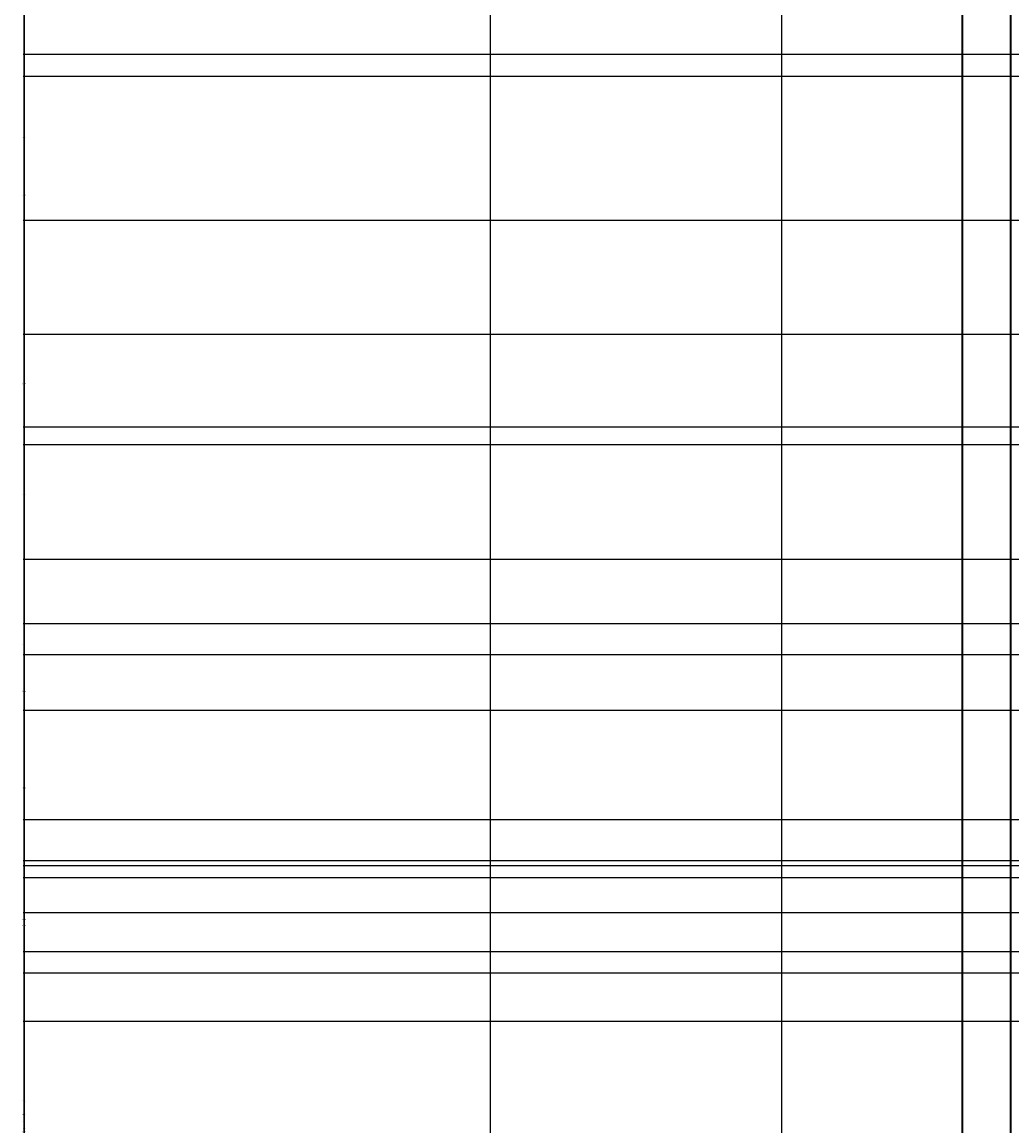
# Model space of a CAD drawing. Units: inches. Extents: x 818 to 1898, y 976 to 2364.
# Tile 9 of 96: x 818 to 1002, y 1668 to 1873. Entities that reach past the tile are written whole.
import ezdxf

# ---------------------------------------------------------------- set-up
doc = ezdxf.new("R2010")
doc.units = ezdxf.units.IN
doc.header["$LTSCALE"] = 5
doc.header["$MEASUREMENT"] = 0
doc.layers.add('A-ANNO-DIMS', color=2, linetype='Continuous', lineweight=18)
doc.layers.add('C-PROP', color=7, linetype='Continuous', lineweight=35)
doc.styles.get("Standard").update_dxf_attribs({"font": 'arial.ttf'})
doc.dimstyles.get("Standard").update_dxf_attribs({"dimtxt": 0.18, "dimasz": 0.18, "dimexe": 0.18, "dimexo": 0.0625, "dimgap": 0.09, "dimtad": 0, "dimtih": 1, "dimtoh": 1, "dimdec": 4, "dimzin": 0, "dimdsep": 46, "dimtxsty": 'Standard', "dimcen": 0.09, "dimadec": 0, "dimazin": 0, "dimtfac": 1, "dimtdec": 4, "dimtofl": 0, "dimtmove": 0, "dimatfit": 3, "dimfxl": 1, "dimtolj": 1, "dimtzin": 0, "dimarcsym": 0})

# ---------------------------------------------------------------- blocks, each defined once
blk = doc.blocks.new('*D59')
at = {"layer": 'A-ANNO-DIMS', "color": 0, "lineweight": -2, "ltscale": 5, "transparency": 16777216}
for p, q in [((1251.64, 2300.39), (818.03, 2300.39)), ((818.21, 2300.21), (818.21, 1669.95)), ((818.21, 1039.32), (818.21, 1669.59)), ((896.05, 1039.14), (818.03, 1039.14))]:
    blk.add_line(p, q, dxfattribs=at)
at = {"layer": 'A-ANNO-DIMS', "color": 0, "ltscale": 5, "transparency": 16777216}
for points in [[(818.18, 2300.21), (818.24, 2300.21), (818.21, 2300.39)], [(818.18, 1039.32), (818.24, 1039.32), (818.21, 1039.14)]]:
    blk.add_solid(points, dxfattribs=at)
at = {"layer": 'Defpoints', "color": 0, "ltscale": 5, "transparency": 16777216}
for p in [(818.21, 2300.39), (1251.71, 2300.39), (896.11, 1039.14)]:
    blk.add_point(p, dxfattribs=at)
at = {"layer": 'A-ANNO-DIMS', "color": 0, "ltscale": 5, "transparency": 16777216, "insert": (818.21, 1669.77), "char_height": 0.18, "attachment_point": 5}
blk.add_mtext('\\A1;1261.2', dxfattribs=at)
blk = doc.blocks.new('*D60')
at = {"layer": 'A-ANNO-DIMS', "color": 0, "lineweight": -2, "ltscale": 5, "transparency": 16777216}
for p, q in [((992.66, 2294.22), (818.03, 2294.22)), ((818.21, 2294.04), (818.21, 1748.77)), ((818.21, 1203.14), (818.21, 1748.41)), ((992.66, 1202.96), (818.03, 1202.96))]:
    blk.add_line(p, q, dxfattribs=at)
at = {"layer": 'A-ANNO-DIMS', "color": 0, "ltscale": 5, "transparency": 16777216}
for points in [[(818.18, 2294.04), (818.24, 2294.04), (818.21, 2294.22)], [(818.18, 1203.14), (818.24, 1203.14), (818.21, 1202.96)]]:
    blk.add_solid(points, dxfattribs=at)
at = {"layer": 'Defpoints', "color": 0, "ltscale": 5, "transparency": 16777216}
for p in [(818.21, 2294.22), (992.73, 2294.22), (992.73, 1202.96)]:
    blk.add_point(p, dxfattribs=at)
at = {"layer": 'A-ANNO-DIMS', "color": 0, "ltscale": 5, "transparency": 16777216, "insert": (818.21, 1748.59), "char_height": 0.18, "attachment_point": 5}
blk.add_mtext('\\A1;1091.3', dxfattribs=at)
blk = doc.blocks.new('*D79')
at = {"layer": 'A-ANNO-DIMS', "color": 0, "lineweight": -2, "ltscale": 5, "transparency": 16777216}
for p, q in [((992.73, 1203.03), (992.73, 2363.87)), ((992.91, 2363.69), (1032.01, 2363.69)), ((1071.55, 2363.69), (1032.44, 2363.69)), ((1071.73, 1203.03), (1071.73, 2363.87))]:
    blk.add_line(p, q, dxfattribs=at)
at = {"layer": 'A-ANNO-DIMS', "color": 0, "ltscale": 5, "transparency": 16777216}
for points in [[(992.91, 2363.72), (992.91, 2363.66), (992.73, 2363.69)], [(1071.55, 2363.72), (1071.55, 2363.66), (1071.73, 2363.69)]]:
    blk.add_solid(points, dxfattribs=at)
at = {"layer": 'Defpoints', "color": 0, "ltscale": 5, "transparency": 16777216}
for p in [(1071.73, 2363.69), (992.73, 1202.96), (1071.73, 1202.96)]:
    blk.add_point(p, dxfattribs=at)
at = {"layer": 'A-ANNO-DIMS', "color": 0, "ltscale": 5, "transparency": 16777216, "insert": (1032.23, 2363.69), "char_height": 0.18, "attachment_point": 5}
blk.add_mtext('\\A1;79', dxfattribs=at)
blk = doc.blocks.new('*D84')
at = {"layer": 'A-ANNO-DIMS', "color": 0, "lineweight": -2, "ltscale": 5, "transparency": 16777216}
for p, q in [((1197.66, 1700.08), (818.03, 1700.08)), ((818.21, 1699.9), (818.21, 1600.76)), ((818.21, 1501.26), (818.21, 1600.4)), ((1197.66, 1501.08), (818.03, 1501.08))]:
    blk.add_line(p, q, dxfattribs=at)
at = {"layer": 'A-ANNO-DIMS', "color": 0, "ltscale": 5, "transparency": 16777216}
for points in [[(818.18, 1699.9), (818.24, 1699.9), (818.21, 1700.08)], [(818.18, 1501.26), (818.24, 1501.26), (818.21, 1501.08)]]:
    blk.add_solid(points, dxfattribs=at)
at = {"layer": 'Defpoints', "color": 0, "ltscale": 5, "transparency": 16777216}
for p in [(818.21, 1700.08), (1197.73, 1700.08), (1197.73, 1501.08)]:
    blk.add_point(p, dxfattribs=at)
at = {"layer": 'A-ANNO-DIMS', "color": 0, "ltscale": 5, "transparency": 16777216, "insert": (818.21, 1600.58), "char_height": 0.18, "attachment_point": 5}
blk.add_mtext('\\A1;199', dxfattribs=at)
blk = doc.blocks.new('*D90')
at = {"layer": 'A-ANNO-DIMS', "color": 0, "lineweight": -2, "ltscale": 5, "transparency": 16777216}
for p, q in [((904.95, 1071.12), (904.95, 2363.87)), ((905.13, 2363.69), (931.67, 2363.69)), ((958.99, 2363.69), (932.45, 2363.69)), ((959.17, 1071.12), (959.17, 2363.87))]:
    blk.add_line(p, q, dxfattribs=at)
at = {"layer": 'A-ANNO-DIMS', "color": 0, "ltscale": 5, "transparency": 16777216}
for points in [[(905.13, 2363.72), (905.13, 2363.66), (904.95, 2363.69)], [(958.99, 2363.72), (958.99, 2363.66), (959.17, 2363.69)]]:
    blk.add_solid(points, dxfattribs=at)
at = {"layer": 'Defpoints', "color": 0, "ltscale": 5, "transparency": 16777216}
for p in [(959.17, 2363.69), (904.95, 1071.06), (959.17, 1071.06)]:
    blk.add_point(p, dxfattribs=at)
at = {"layer": 'A-ANNO-DIMS', "color": 0, "ltscale": 5, "transparency": 16777216, "insert": (932.06, 2363.69), "char_height": 0.18, "attachment_point": 5}
blk.add_mtext('\\A1;54.22', dxfattribs=at)
blk = doc.blocks.new('*D91')
at = {"layer": 'A-ANNO-DIMS', "color": 0, "lineweight": -2, "ltscale": 5, "transparency": 16777216}
for p, q in [((959.17, 1071.12), (959.17, 2363.87)), ((959.35, 2363.69), (985.8, 2363.69)), ((1013.04, 2363.69), (986.59, 2363.69)), ((1013.22, 1071.12), (1013.22, 2363.87))]:
    blk.add_line(p, q, dxfattribs=at)
at = {"layer": 'A-ANNO-DIMS', "color": 0, "ltscale": 5, "transparency": 16777216}
for points in [[(959.35, 2363.72), (959.35, 2363.66), (959.17, 2363.69)], [(1013.04, 2363.72), (1013.04, 2363.66), (1013.22, 2363.69)]]:
    blk.add_solid(points, dxfattribs=at)
at = {"layer": 'Defpoints', "color": 0, "ltscale": 5, "transparency": 16777216}
for p in [(1013.22, 2363.69), (959.17, 1071.06), (1013.22, 1071.06)]:
    blk.add_point(p, dxfattribs=at)
at = {"layer": 'A-ANNO-DIMS', "color": 0, "ltscale": 5, "transparency": 16777216, "insert": (986.2, 2363.69), "char_height": 0.18, "attachment_point": 5}
blk.add_mtext('\\A1;54.04', dxfattribs=at)
blk = doc.blocks.new('*D119')
at = {"layer": 'A-ANNO-DIMS', "color": 0, "lineweight": -2, "ltscale": 5, "transparency": 16777216}
for p, q in [((1766.29, 1716.99), (818.03, 1716.99)), ((818.21, 1716.81), (818.21, 1672.43)), ((818.21, 1627.69), (818.21, 1672.06)), ((1766.29, 1627.51), (818.03, 1627.51))]:
    blk.add_line(p, q, dxfattribs=at)
at = {"layer": 'A-ANNO-DIMS', "color": 0, "ltscale": 5, "transparency": 16777216}
for points in [[(818.18, 1716.81), (818.24, 1716.81), (818.21, 1716.99)], [(818.18, 1627.69), (818.24, 1627.69), (818.21, 1627.51)]]:
    blk.add_solid(points, dxfattribs=at)
at = {"layer": 'Defpoints', "color": 0, "ltscale": 5, "transparency": 16777216}
for p in [(818.21, 1716.99), (1766.35, 1716.99), (1766.35, 1627.51)]:
    blk.add_point(p, dxfattribs=at)
at = {"layer": 'A-ANNO-DIMS', "color": 0, "ltscale": 5, "transparency": 16777216, "insert": (818.21, 1672.25), "char_height": 0.18, "attachment_point": 5}
blk.add_mtext('\\A1;89.48', dxfattribs=at)
blk = doc.blocks.new('*D120')
at = {"layer": 'A-ANNO-DIMS', "color": 0, "lineweight": -2, "ltscale": 5, "transparency": 16777216}
for p, q in [((1766.29, 1797.72), (818.03, 1797.72)), ((818.21, 1797.54), (818.21, 1757.53)), ((818.21, 1717.17), (818.21, 1757.17)), ((1766.29, 1716.99), (818.03, 1716.99))]:
    blk.add_line(p, q, dxfattribs=at)
at = {"layer": 'A-ANNO-DIMS', "color": 0, "ltscale": 5, "transparency": 16777216}
for points in [[(818.18, 1797.54), (818.24, 1797.54), (818.21, 1797.72)], [(818.18, 1717.17), (818.24, 1717.17), (818.21, 1716.99)]]:
    blk.add_solid(points, dxfattribs=at)
at = {"layer": 'Defpoints', "color": 0, "ltscale": 5, "transparency": 16777216}
for p in [(818.21, 1797.72), (1766.35, 1797.72), (1766.35, 1716.99)]:
    blk.add_point(p, dxfattribs=at)
at = {"layer": 'A-ANNO-DIMS', "color": 0, "ltscale": 5, "transparency": 16777216, "insert": (818.21, 1757.35), "char_height": 0.18, "attachment_point": 5}
blk.add_mtext('\\A1;80.73', dxfattribs=at)
blk = doc.blocks.new('*D121')
at = {"layer": 'A-ANNO-DIMS', "color": 0, "lineweight": -2, "ltscale": 5, "transparency": 16777216}
for p, q in [((1766.29, 1884.2), (818.03, 1884.2)), ((818.21, 1884.02), (818.21, 1841.14)), ((818.21, 1797.9), (818.21, 1840.78)), ((1766.29, 1797.72), (818.03, 1797.72))]:
    blk.add_line(p, q, dxfattribs=at)
at = {"layer": 'A-ANNO-DIMS', "color": 0, "ltscale": 5, "transparency": 16777216}
for points in [[(818.18, 1884.02), (818.24, 1884.02), (818.21, 1884.2)], [(818.18, 1797.9), (818.24, 1797.9), (818.21, 1797.72)]]:
    blk.add_solid(points, dxfattribs=at)
at = {"layer": 'Defpoints', "color": 0, "ltscale": 5, "transparency": 16777216}
for p in [(818.21, 1884.2), (1766.35, 1884.2), (1766.35, 1797.72)]:
    blk.add_point(p, dxfattribs=at)
at = {"layer": 'A-ANNO-DIMS', "color": 0, "ltscale": 5, "transparency": 16777216, "insert": (818.21, 1840.96), "char_height": 0.18, "attachment_point": 5}
blk.add_mtext('\\A1;86.49', dxfattribs=at)
blk = doc.blocks.new('*D124')
at = {"layer": 'A-ANNO-DIMS', "color": 0, "lineweight": -2, "ltscale": 5, "transparency": 16777216}
for p, q in [((1131.7, 1974.57), (818.03, 1974.57)), ((818.21, 1974.39), (818.21, 1884.68)), ((818.21, 1794.61), (818.21, 1884.32)), ((1138.44, 1794.43), (818.03, 1794.43))]:
    blk.add_line(p, q, dxfattribs=at)
at = {"layer": 'A-ANNO-DIMS', "color": 0, "ltscale": 5, "transparency": 16777216}
for points in [[(818.18, 1974.39), (818.24, 1974.39), (818.21, 1974.57)], [(818.18, 1794.61), (818.24, 1794.61), (818.21, 1794.43)]]:
    blk.add_solid(points, dxfattribs=at)
at = {"layer": 'Defpoints', "color": 0, "ltscale": 5, "transparency": 16777216}
for p in [(818.21, 1974.57), (1131.77, 1974.57), (1138.5, 1794.43)]:
    blk.add_point(p, dxfattribs=at)
at = {"layer": 'A-ANNO-DIMS', "color": 0, "ltscale": 5, "transparency": 16777216, "insert": (818.21, 1884.5), "char_height": 0.18, "attachment_point": 5}
blk.add_mtext('\\A1;180.14', dxfattribs=at)
blk = doc.blocks.new('*D130')
at = {"layer": 'A-ANNO-DIMS', "color": 0, "lineweight": -2, "ltscale": 5, "transparency": 16777216}
for p, q in [((1044.78, 1724.63), (818.03, 1724.63)), ((818.21, 1724.45), (818.21, 1666.75)), ((818.21, 1608.69), (818.21, 1666.39)), ((1044.78, 1608.51), (818.03, 1608.51))]:
    blk.add_line(p, q, dxfattribs=at)
at = {"layer": 'A-ANNO-DIMS', "color": 0, "ltscale": 5, "transparency": 16777216}
for points in [[(818.18, 1724.45), (818.24, 1724.45), (818.21, 1724.63)], [(818.18, 1608.69), (818.24, 1608.69), (818.21, 1608.51)]]:
    blk.add_solid(points, dxfattribs=at)
at = {"layer": 'Defpoints', "color": 0, "ltscale": 5, "transparency": 16777216}
for p in [(818.21, 1724.63), (1044.85, 1724.63), (1044.85, 1608.51)]:
    blk.add_point(p, dxfattribs=at)
at = {"layer": 'A-ANNO-DIMS', "color": 0, "ltscale": 5, "transparency": 16777216, "insert": (818.21, 1666.57), "char_height": 0.18, "attachment_point": 5}
blk.add_mtext('\\A1;116.12', dxfattribs=at)
blk = doc.blocks.new('*D131')
at = {"layer": 'A-ANNO-DIMS', "color": 0, "lineweight": -2, "ltscale": 5, "transparency": 16777216}
for p, q in [((1043.71, 1886.9), (818.03, 1886.9)), ((818.21, 1886.72), (818.21, 1805.95)), ((818.21, 1724.81), (818.21, 1805.58)), ((1044.78, 1724.63), (818.03, 1724.63))]:
    blk.add_line(p, q, dxfattribs=at)
at = {"layer": 'A-ANNO-DIMS', "color": 0, "ltscale": 5, "transparency": 16777216}
for points in [[(818.18, 1886.72), (818.24, 1886.72), (818.21, 1886.9)], [(818.18, 1724.81), (818.24, 1724.81), (818.21, 1724.63)]]:
    blk.add_solid(points, dxfattribs=at)
at = {"layer": 'Defpoints', "color": 0, "ltscale": 5, "transparency": 16777216}
for p in [(818.21, 1886.9), (1043.77, 1886.9), (1044.85, 1724.63)]:
    blk.add_point(p, dxfattribs=at)
at = {"layer": 'A-ANNO-DIMS', "color": 0, "ltscale": 5, "transparency": 16777216, "insert": (818.21, 1805.77), "char_height": 0.18, "attachment_point": 5}
blk.add_mtext('\\A1;162.27', dxfattribs=at)
blk = doc.blocks.new('*D162')
at = {"layer": 'A-ANNO-DIMS', "color": 0, "lineweight": -2, "ltscale": 5, "transparency": 16777216}
for p, q in [((1429.16, 1876.08), (818.03, 1876.08)), ((818.21, 1875.9), (818.21, 1871.76)), ((818.21, 1867.26), (818.21, 1871.4)), ((1429.16, 1867.08), (818.03, 1867.08))]:
    blk.add_line(p, q, dxfattribs=at)
at = {"layer": 'A-ANNO-DIMS', "color": 0, "ltscale": 5, "transparency": 16777216}
for points in [[(818.18, 1875.9), (818.24, 1875.9), (818.21, 1876.08)], [(818.18, 1867.26), (818.24, 1867.26), (818.21, 1867.08)]]:
    blk.add_solid(points, dxfattribs=at)
at = {"layer": 'Defpoints', "color": 0, "ltscale": 5, "transparency": 16777216}
for p in [(1429.23, 1876.08), (818.21, 1867.08), (1429.23, 1867.08)]:
    blk.add_point(p, dxfattribs=at)
at = {"layer": 'A-ANNO-DIMS', "color": 0, "ltscale": 5, "transparency": 16777216, "insert": (818.21, 1871.58), "char_height": 0.18, "attachment_point": 5}
blk.add_mtext('\\A1;9', dxfattribs=at)
blk = doc.blocks.new('*D176')
at = {"layer": 'A-ANNO-DIMS', "color": 0, "lineweight": -2, "ltscale": 5, "transparency": 16777216}
for p, q in [((1559.66, 1687.08), (818.03, 1687.08)), ((818.21, 1686.9), (818.21, 1667.51)), ((818.21, 1647.76), (818.21, 1667.15)), ((1559.66, 1647.58), (818.03, 1647.58))]:
    blk.add_line(p, q, dxfattribs=at)
at = {"layer": 'A-ANNO-DIMS', "color": 0, "ltscale": 5, "transparency": 16777216}
for points in [[(818.18, 1686.9), (818.24, 1686.9), (818.21, 1687.08)], [(818.18, 1647.76), (818.24, 1647.76), (818.21, 1647.58)]]:
    blk.add_solid(points, dxfattribs=at)
at = {"layer": 'Defpoints', "color": 0, "ltscale": 5, "transparency": 16777216}
for p in [(1559.73, 1687.08), (818.21, 1647.58), (1559.73, 1647.58)]:
    blk.add_point(p, dxfattribs=at)
at = {"layer": 'A-ANNO-DIMS', "color": 0, "ltscale": 5, "transparency": 16777216, "insert": (818.21, 1667.33), "char_height": 0.18, "attachment_point": 5}
blk.add_mtext('\\A1;39.5', dxfattribs=at)
blk = doc.blocks.new('*D215')
at = {"layer": 'A-ANNO-DIMS', "color": 0, "lineweight": -2, "ltscale": 5, "transparency": 16777216}
for p, q in [((1590.66, 1876.08), (818.03, 1876.08)), ((818.21, 1875.9), (818.21, 1781.76)), ((818.21, 1687.26), (818.21, 1781.4)), ((1511.66, 1687.08), (818.03, 1687.08))]:
    blk.add_line(p, q, dxfattribs=at)
at = {"layer": 'A-ANNO-DIMS', "color": 0, "ltscale": 5, "transparency": 16777216}
for points in [[(818.18, 1875.9), (818.24, 1875.9), (818.21, 1876.08)], [(818.18, 1687.26), (818.24, 1687.26), (818.21, 1687.08)]]:
    blk.add_solid(points, dxfattribs=at)
at = {"layer": 'Defpoints', "color": 0, "ltscale": 5, "transparency": 16777216}
for p in [(818.21, 1876.08), (1590.73, 1876.08), (1511.73, 1687.08)]:
    blk.add_point(p, dxfattribs=at)
at = {"layer": 'A-ANNO-DIMS', "color": 0, "ltscale": 5, "transparency": 16777216, "insert": (818.21, 1781.58), "char_height": 0.18, "attachment_point": 5}
blk.add_mtext('\\A1;189', dxfattribs=at)
blk = doc.blocks.new('*D220')
at = {"layer": 'A-ANNO-DIMS', "color": 0, "lineweight": -2, "ltscale": 5, "transparency": 16777216}
for p, q in [((1520.66, 1773.08), (818.03, 1773.08)), ((818.21, 1772.9), (818.21, 1767.26)), ((818.21, 1761.26), (818.21, 1766.9)), ((1520.66, 1761.08), (818.03, 1761.08))]:
    blk.add_line(p, q, dxfattribs=at)
at = {"layer": 'A-ANNO-DIMS', "color": 0, "ltscale": 5, "transparency": 16777216}
for points in [[(818.18, 1772.9), (818.24, 1772.9), (818.21, 1773.08)], [(818.18, 1761.26), (818.24, 1761.26), (818.21, 1761.08)]]:
    blk.add_solid(points, dxfattribs=at)
at = {"layer": 'Defpoints', "color": 0, "ltscale": 5, "transparency": 16777216}
for p in [(818.21, 1773.08), (1520.73, 1773.08), (1520.73, 1761.08)]:
    blk.add_point(p, dxfattribs=at)
at = {"layer": 'A-ANNO-DIMS', "color": 0, "ltscale": 5, "transparency": 16777216, "insert": (818.21, 1767.08), "char_height": 0.18, "attachment_point": 5}
blk.add_mtext('\\A1;12', dxfattribs=at)
blk = doc.blocks.new('*D222')
at = {"layer": 'A-ANNO-DIMS', "color": 0, "lineweight": -2, "ltscale": 5, "transparency": 16777216}
for p, q in [((1511.66, 1744.97), (818.03, 1744.97)), ((818.21, 1744.79), (818.21, 1730.69)), ((818.21, 1716.23), (818.21, 1730.33)), ((1511.66, 1716.05), (818.03, 1716.05))]:
    blk.add_line(p, q, dxfattribs=at)
at = {"layer": 'A-ANNO-DIMS', "color": 0, "ltscale": 5, "transparency": 16777216}
for points in [[(818.18, 1744.79), (818.24, 1744.79), (818.21, 1744.97)], [(818.18, 1716.23), (818.24, 1716.23), (818.21, 1716.05)]]:
    blk.add_solid(points, dxfattribs=at)
at = {"layer": 'Defpoints', "color": 0, "ltscale": 5, "transparency": 16777216}
for p in [(818.21, 1744.97), (1511.73, 1744.97), (1511.73, 1716.05)]:
    blk.add_point(p, dxfattribs=at)
at = {"layer": 'A-ANNO-DIMS', "color": 0, "ltscale": 5, "transparency": 16777216, "insert": (818.21, 1730.51), "char_height": 0.18, "attachment_point": 5}
blk.add_mtext('\\A1;28.926', dxfattribs=at)
blk = doc.blocks.new('*D223')
at = {"layer": 'A-ANNO-DIMS', "color": 0, "lineweight": -2, "ltscale": 5, "transparency": 16777216}
for p, q in [((1511.66, 1716.05), (818.03, 1716.05)), ((818.21, 1715.87), (818.21, 1706.24)), ((818.21, 1696.26), (818.21, 1705.88)), ((1511.66, 1696.08), (818.03, 1696.08))]:
    blk.add_line(p, q, dxfattribs=at)
at = {"layer": 'A-ANNO-DIMS', "color": 0, "ltscale": 5, "transparency": 16777216}
for points in [[(818.18, 1715.87), (818.24, 1715.87), (818.21, 1716.05)], [(818.18, 1696.26), (818.24, 1696.26), (818.21, 1696.08)]]:
    blk.add_solid(points, dxfattribs=at)
at = {"layer": 'Defpoints', "color": 0, "ltscale": 5, "transparency": 16777216}
for p in [(818.21, 1716.05), (1511.73, 1716.05), (1511.73, 1696.08)]:
    blk.add_point(p, dxfattribs=at)
at = {"layer": 'A-ANNO-DIMS', "color": 0, "ltscale": 5, "transparency": 16777216, "insert": (818.21, 1706.06), "char_height": 0.18, "attachment_point": 5}
blk.add_mtext('\\A1;19.967', dxfattribs=at)
blk = doc.blocks.new('*D227')
at = {"layer": 'A-ANNO-DIMS', "color": 0, "lineweight": -2, "ltscale": 5, "transparency": 16777216}
for p, q in [((1595.66, 1867.08), (818.03, 1867.08)), ((818.21, 1866.9), (818.21, 1851.81)), ((818.21, 1836.36), (818.21, 1851.45)), ((1594.66, 1836.18), (818.03, 1836.18))]:
    blk.add_line(p, q, dxfattribs=at)
at = {"layer": 'A-ANNO-DIMS', "color": 0, "ltscale": 5, "transparency": 16777216}
for points in [[(818.18, 1866.9), (818.24, 1866.9), (818.21, 1867.08)], [(818.18, 1836.36), (818.24, 1836.36), (818.21, 1836.18)]]:
    blk.add_solid(points, dxfattribs=at)
at = {"layer": 'Defpoints', "color": 0, "ltscale": 5, "transparency": 16777216}
for p in [(818.21, 1867.08), (1595.73, 1867.08), (1594.73, 1836.18)]:
    blk.add_point(p, dxfattribs=at)
at = {"layer": 'A-ANNO-DIMS', "color": 0, "ltscale": 5, "transparency": 16777216, "insert": (818.21, 1851.63), "char_height": 0.18, "attachment_point": 5}
blk.add_mtext('\\A1;30.894', dxfattribs=at)
blk = doc.blocks.new('*D246')
at = {"layer": 'A-ANNO-DIMS', "color": 0, "lineweight": -2, "ltscale": 5, "transparency": 16777216}
for p, q in [((1258.66, 1755.33), (818.03, 1755.33)), ((818.21, 1755.15), (818.21, 1731.51)), ((818.21, 1707.51), (818.21, 1731.15)), ((1258.66, 1707.33), (818.03, 1707.33))]:
    blk.add_line(p, q, dxfattribs=at)
at = {"layer": 'A-ANNO-DIMS', "color": 0, "ltscale": 5, "transparency": 16777216}
for points in [[(818.18, 1755.15), (818.24, 1755.15), (818.21, 1755.33)], [(818.18, 1707.51), (818.24, 1707.51), (818.21, 1707.33)]]:
    blk.add_solid(points, dxfattribs=at)
at = {"layer": 'Defpoints', "color": 0, "ltscale": 5, "transparency": 16777216}
for p in [(818.21, 1755.33), (1258.73, 1755.33), (1258.73, 1707.33)]:
    blk.add_point(p, dxfattribs=at)
at = {"layer": 'A-ANNO-DIMS', "color": 0, "ltscale": 5, "transparency": 16777216, "insert": (818.21, 1731.33), "char_height": 0.18, "attachment_point": 5}
blk.add_mtext('\\A1;48', dxfattribs=at)
blk = doc.blocks.new('*D247')
at = {"layer": 'A-ANNO-DIMS', "color": 0, "lineweight": -2, "ltscale": 5, "transparency": 16777216}
for p, q in [((1258.66, 1862.97), (818.03, 1862.97)), ((818.21, 1862.79), (818.21, 1839.15)), ((818.21, 1815.15), (818.21, 1838.78)), ((1258.66, 1814.97), (818.03, 1814.97))]:
    blk.add_line(p, q, dxfattribs=at)
at = {"layer": 'A-ANNO-DIMS', "color": 0, "ltscale": 5, "transparency": 16777216}
for points in [[(818.18, 1862.79), (818.24, 1862.79), (818.21, 1862.97)], [(818.18, 1815.15), (818.24, 1815.15), (818.21, 1814.97)]]:
    blk.add_solid(points, dxfattribs=at)
at = {"layer": 'Defpoints', "color": 0, "ltscale": 5, "transparency": 16777216}
for p in [(818.21, 1862.97), (1258.73, 1862.97), (1258.73, 1814.97)]:
    blk.add_point(p, dxfattribs=at)
at = {"layer": 'A-ANNO-DIMS', "color": 0, "ltscale": 5, "transparency": 16777216, "insert": (818.21, 1838.97), "char_height": 0.18, "attachment_point": 5}
blk.add_mtext('\\A1;48', dxfattribs=at)
blk = doc.blocks.new('*D249')
at = {"layer": 'A-ANNO-DIMS', "color": 0, "lineweight": -2, "ltscale": 5, "transparency": 16777216}
for p, q in [((1258.66, 1814.97), (818.03, 1814.97)), ((818.21, 1814.79), (818.21, 1785.33)), ((818.21, 1755.51), (818.21, 1784.97)), ((1258.66, 1755.33), (818.03, 1755.33))]:
    blk.add_line(p, q, dxfattribs=at)
at = {"layer": 'A-ANNO-DIMS', "color": 0, "ltscale": 5, "transparency": 16777216}
for points in [[(818.18, 1814.79), (818.24, 1814.79), (818.21, 1814.97)], [(818.18, 1755.51), (818.24, 1755.51), (818.21, 1755.33)]]:
    blk.add_solid(points, dxfattribs=at)
at = {"layer": 'Defpoints', "color": 0, "ltscale": 5, "transparency": 16777216}
for p in [(818.21, 1814.97), (1258.73, 1814.97), (1258.73, 1755.33)]:
    blk.add_point(p, dxfattribs=at)
at = {"layer": 'A-ANNO-DIMS', "color": 0, "ltscale": 5, "transparency": 16777216, "insert": (818.21, 1785.15), "char_height": 0.18, "attachment_point": 5}
blk.add_mtext('\\A1;59.63', dxfattribs=at)
blk = doc.blocks.new('*D277')
at = {"layer": 'A-ANNO-DIMS', "color": 0, "lineweight": -2, "ltscale": 5, "transparency": 16777216}
for p, q in [((1251.87, 1687.08), (818.03, 1687.08)), ((818.21, 1686.9), (818.21, 1668.7)), ((818.21, 1650.13), (818.21, 1668.33)), ((1256.59, 1649.95), (818.03, 1649.95))]:
    blk.add_line(p, q, dxfattribs=at)
at = {"layer": 'A-ANNO-DIMS', "color": 0, "ltscale": 5, "transparency": 16777216}
for points in [[(818.18, 1686.9), (818.24, 1686.9), (818.21, 1687.08)], [(818.18, 1650.13), (818.24, 1650.13), (818.21, 1649.95)]]:
    blk.add_solid(points, dxfattribs=at)
at = {"layer": 'Defpoints', "color": 0, "ltscale": 5, "transparency": 16777216}
for p in [(818.21, 1687.08), (1251.93, 1687.08), (1256.65, 1649.95)]:
    blk.add_point(p, dxfattribs=at)
at = {"layer": 'A-ANNO-DIMS', "color": 0, "ltscale": 5, "transparency": 16777216, "insert": (818.21, 1668.52), "char_height": 0.18, "attachment_point": 5}
blk.add_mtext('\\A1;37.13', dxfattribs=at)
blk = doc.blocks.new('*D289')
at = {"layer": 'A-ANNO-DIMS', "color": 0, "lineweight": -2, "ltscale": 5, "transparency": 16777216}
for p, q in [((1279.06, 1713.82), (818.03, 1713.82)), ((818.21, 1713.64), (818.21, 1705.13)), ((818.21, 1696.26), (818.21, 1704.77)), ((1267.66, 1696.08), (818.03, 1696.08))]:
    blk.add_line(p, q, dxfattribs=at)
at = {"layer": 'A-ANNO-DIMS', "color": 0, "ltscale": 5, "transparency": 16777216}
for points in [[(818.18, 1713.64), (818.24, 1713.64), (818.21, 1713.82)], [(818.18, 1696.26), (818.24, 1696.26), (818.21, 1696.08)]]:
    blk.add_solid(points, dxfattribs=at)
at = {"layer": 'Defpoints', "color": 0, "ltscale": 5, "transparency": 16777216}
for p in [(1279.13, 1713.82), (818.21, 1696.08), (1267.73, 1696.08)]:
    blk.add_point(p, dxfattribs=at)
at = {"layer": 'A-ANNO-DIMS', "color": 0, "ltscale": 5, "transparency": 16777216, "insert": (818.21, 1704.95), "char_height": 0.18, "attachment_point": 5}
blk.add_mtext('\\A1;17.74', dxfattribs=at)

msp = doc.modelspace()

# ---------------------------------------------------------------- linework, layer by layer
at = {"layer": 'C-PROP'}
for p, q in [((992.7251, 2294.2171), (992.7251, 1202.9642)), ((1001.7252, 2285.2171), (1001.7252, 1211.9642))]:
    msp.add_line(p, q, dxfattribs=at)

# ---------------------------------------------------------------- dimensions: what is measured, and where the dimension line sits
at = {"layer": 'A-ANNO-DIMS', "ltscale": 5}
for base, p1, p2, override, picture, middle in [((959.1737, 2363.6929), (904.9504, 1071.0552), (959.1737, 1071.0552), {"dimdec": 2, "dimlfac": 1, "dimrnd": 0, "dimzin": 0, "dimdsep": 46, "dimlunit": 2}, '*D90', (932.062, 2363.6929)), ((1013.2176, 2363.6929), (959.1737, 1071.0552), (1013.2176, 1071.0552), {"dimdec": 2, "dimlfac": 1, "dimrnd": 0, "dimzin": 0, "dimdsep": 46, "dimlunit": 2}, '*D91', (986.1956, 2363.6929)), ((1071.7251, 2363.6929), (992.7251, 1202.9642), (1071.7251, 1202.9642), {"dimdec": 0, "dimlfac": 1, "dimrnd": 0, "dimzin": 0, "dimdsep": 46, "dimlunit": 2}, '*D79', (1032.2251, 2363.6929))]:
    dim = msp.add_linear_dim(base=base, p1=p1, p2=p2, dimstyle='Standard', override=override, dxfattribs=at)
    dim.commit()
    dim.dimension.update_dxf_attribs({"geometry": picture, "text_midpoint": middle})
for base, p1, p2, override, picture, middle in [((818.2059, 2300.3929), (896.1138, 1039.1433), (1251.7057, 2300.3929), {"dimdec": 1, "dimlfac": 1, "dimrnd": 0, "dimzin": 0, "dimdsep": 46, "dimlunit": 2}, '*D59', (818.2059, 1669.7681)), ((818.2059, 2294.2171), (992.7251, 1202.9642), (992.7251, 2294.2171), {"dimdec": 1, "dimlfac": 1, "dimrnd": 0, "dimzin": 0, "dimdsep": 46, "dimlunit": 2}, '*D60', (818.2059, 1748.5907)), ((818.2059, 1974.5735), (1138.5041, 1794.4325), (1131.7651, 1974.5735), {"dimdec": 2, "dimlfac": 1, "dimrnd": 0, "dimzin": 0, "dimdsep": 46, "dimlunit": 2}, '*D124', (818.2059, 1884.503)), ((818.2059, 1886.9018), (1044.8463, 1724.63), (1043.7685, 1886.9018), {"dimdec": 2, "dimlfac": 1, "dimrnd": 0, "dimzin": 0, "dimdsep": 46, "dimlunit": 2}, '*D131', (818.2059, 1805.7659)), ((818.2059, 1884.2031), (1766.3524, 1797.7165), (1766.3524, 1884.2031), {"dimdec": 2, "dimlfac": 1, "dimrnd": 0, "dimzin": 0, "dimdsep": 46, "dimlunit": 2}, '*D121', (818.2059, 1840.9598)), ((818.2059, 1876.0782), (1511.7251, 1687.0782), (1590.7251, 1876.0782), {"dimdec": 0, "dimlfac": 1, "dimrnd": 0, "dimzin": 0, "dimdsep": 46, "dimlunit": 2}, '*D215', (818.2059, 1781.5782)), ((818.2059, 1867.0782), (1429.2251, 1876.0782), (1429.2251, 1867.0782), {"dimdec": 0, "dimlfac": 1, "dimrnd": 0, "dimzin": 0, "dimdsep": 46, "dimlunit": 2}, '*D162', (818.2059, 1871.5782)), ((818.2059, 1867.0782), (1594.7251, 1836.1844), (1595.7251, 1867.0782), {"dimdec": 3, "dimlfac": 1, "dimrnd": 0, "dimzin": 0, "dimdsep": 46, "dimlunit": 2}, '*D227', (818.2059, 1851.6313)), ((818.2059, 1862.9652), (1258.7251, 1814.9652), (1258.7251, 1862.9652), {"dimdec": 0, "dimlfac": 1, "dimrnd": 0, "dimzin": 0, "dimdsep": 46, "dimlunit": 2}, '*D247', (818.2059, 1838.9652)), ((818.2059, 1814.9652), (1258.7251, 1755.3321), (1258.7251, 1814.9652), {"dimdec": 2, "dimlfac": 1, "dimrnd": 0, "dimzin": 0, "dimdsep": 46, "dimlunit": 2}, '*D249', (818.2059, 1785.1486)), ((818.2059, 1797.7165), (1766.3524, 1716.9866), (1766.3524, 1797.7165), {"dimdec": 2, "dimlfac": 1, "dimrnd": 0, "dimzin": 0, "dimdsep": 46, "dimlunit": 2}, '*D120', (818.2059, 1757.3516)), ((818.2059, 1773.0782), (1520.7251, 1761.0782), (1520.7251, 1773.0782), {"dimdec": 0, "dimlfac": 1, "dimrnd": 0, "dimzin": 0, "dimdsep": 46, "dimlunit": 2}, '*D220', (818.2059, 1767.0782)), ((818.2059, 1755.3321), (1258.7251, 1707.3321), (1258.7251, 1755.3321), {"dimdec": 0, "dimlfac": 1, "dimrnd": 0, "dimzin": 0, "dimdsep": 46, "dimlunit": 2}, '*D246', (818.2059, 1731.3321)), ((818.2059, 1744.9714), (1511.7251, 1716.0454), (1511.7251, 1744.9714), {"dimdec": 3, "dimlfac": 1, "dimrnd": 0, "dimzin": 0, "dimdsep": 46, "dimlunit": 2}, '*D222', (818.2059, 1730.5084)), ((818.2059, 1724.63), (1044.8463, 1608.5116), (1044.8463, 1724.63), {"dimdec": 2, "dimlfac": 1, "dimrnd": 0, "dimzin": 0, "dimdsep": 46, "dimlunit": 2}, '*D130', (818.2059, 1666.5708)), ((818.2059, 1716.0454), (1511.7251, 1696.0782), (1511.7251, 1716.0454), {"dimdec": 3, "dimlfac": 1, "dimrnd": 0, "dimzin": 0, "dimdsep": 46, "dimlunit": 2}, '*D223', (818.2059, 1706.0618)), ((818.2059, 1716.9866), (1766.3524, 1627.5052), (1766.3524, 1716.9866), {"dimdec": 2, "dimlfac": 1, "dimrnd": 0, "dimzin": 0, "dimdsep": 46, "dimlunit": 2}, '*D119', (818.2059, 1672.2459)), ((818.2059, 1696.0782), (1279.1253, 1713.8174), (1267.7251, 1696.0782), {"dimdec": 2, "dimlfac": 1, "dimrnd": 0, "dimzin": 0, "dimdsep": 46, "dimlunit": 2}, '*D289', (818.2059, 1704.9478)), ((818.2059, 1700.0782), (1197.7251, 1501.0782), (1197.7251, 1700.0782), {"dimdec": 0, "dimlfac": 1, "dimrnd": 0, "dimzin": 0, "dimdsep": 46, "dimlunit": 2}, '*D84', (818.2059, 1600.5782)), ((818.2059, 1687.0782), (1256.6519, 1649.9518), (1251.9333, 1687.0782), {"dimdec": 2, "dimlfac": 1, "dimrnd": 0, "dimzin": 0, "dimdsep": 46, "dimlunit": 2}, '*D277', (818.2059, 1668.515)), ((818.2059, 1647.5782), (1559.7251, 1687.0782), (1559.7251, 1647.5782), {"dimdec": 1, "dimlfac": 1, "dimrnd": 0, "dimzin": 0, "dimdsep": 46, "dimlunit": 2}, '*D176', (818.2059, 1667.3282))]:
    dim = msp.add_linear_dim(base=base, p1=p1, p2=p2, angle=90, dimstyle='Standard', override=override, dxfattribs=at)
    dim.commit()
    dim.dimension.update_dxf_attribs({"geometry": picture, "text_midpoint": middle})

doc.saveas('drawing.dxf')
